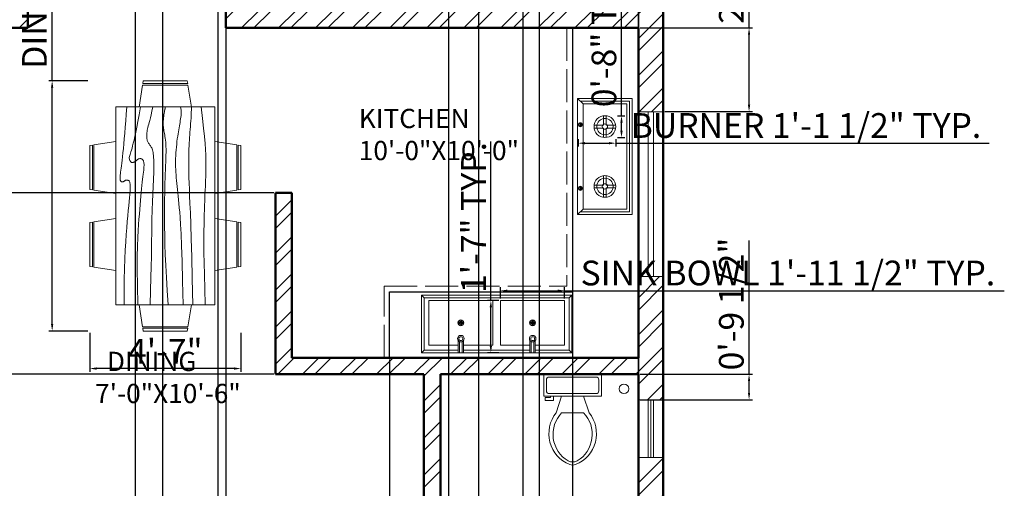
# Model space of a CAD drawing. Units: inches. Extents: x 1104 to 1745, y 678 to 1361.
# Tile 3 of 4: x 1387 to 1745, y 910 to 1080. Entities that reach past the tile are written whole.
import ezdxf

# ---------------------------------------------------------------- set-up
doc = ezdxf.new("R2010")
doc.units = ezdxf.units.IN
doc.linetypes.add('ACAD_ISO02W100', pattern=[15, 12, -3])
for name, color, linetype, lineweight in [('A-ANNO-DIMS', 2, 'Continuous', 18), ('A-AREA-IDEN', 7, 'Continuous', 25), ('A-EQPM', 9, 'Continuous', 18), ('A-FLOR-CASE', 32, 'Continuous', 25), ('A-FLOR-CASE-OVHD', 32, 'ACAD_ISO02W100', 18), ('A-FLOR-FIXT', 8, 'Continuous', 18), ('A-FURN', 8, 'Continuous', 18), ('A-WALL', 7, 'Continuous', 50), ('A-WALL-PATT', 252, 'ACAD_ISO02W100', 13)]:
    doc.layers.add(name, color=color, linetype=linetype, lineweight=lineweight)
doc.layers.add('A-GLAZ', color=244, linetype='Continuous', lineweight=18, true_color=0x991b1e)
doc.styles.get("Standard").update_dxf_attribs({"font": 'arial.ttf'})
doc.dimstyles.new('ISO-25', dxfattribs={"dimtxt": 9, "dimasz": 2.5, "dimexe": 1.25, "dimexo": 0.625, "dimtad": 1, "dimlunit": 3, "dimtxsty": 'Standard', "dimcen": 2.5, "dimadec": 0, "dimazin": 0, "dimtfac": 1, "dimtmove": 0, "dimatfit": 3, "dimfxl": 1, "dimarcsym": 0})

# ---------------------------------------------------------------- blocks, each defined once
blk = doc.blocks.new('*U14')
for p, q in [((9.5, -6), (9.5, -2)), ((-10, -8.5), (-8, -8.5)), ((-10, -9.5), (-10, -8.5)), ((-7, -9.5), (-10, -9.5)), ((-8, -8.5), (-8, -8)), ((-7, -8), (-7, -9.5)), ((-4, -8), (-6, -14)), ((4, -8), (6, -14)), ((4, -14), (-4, -14))]:
    blk.add_line(p, q)
blk.add_lwpolyline([(10.5, -8), (10.5, 0), (-10.5, 0), (-10.5, -8)], close=True)
for points in [[(-9.5, -2), (-9.5, -6)], [(8.5, -1), (-8.5, -1)], [(-8.5, -7), (8.5, -7)]]:
    blk.add_lwpolyline(points)
for centre, radius, start, end in [((-8.62, -1.88), 0.884, 81.8699, 188.1301), ((8.62, -1.88), 0.884, 351.8699, 98.1301), ((-8.62, -6.12), 0.884, 171.8699, 278.1301), ((8.62, -6.12), 0.884, 261.8699, 8.1301), ((3.52, -21.58), 12.17, 141.4691, 247.9714), ((4.2, -21.82), 11.33, 136.3677, 238.9468), ((-3.52, -21.58), 12.17, 292.0284, 38.5307), ((-4.2, -21.82), 11.33, 301.053, 43.6321), ((0, -27.88), 4, 245.7318, 294.2682), ((0, -29), 4, 254.8605, 285.1395)]:
    blk.add_arc(centre, radius, start, end)
blk = doc.blocks.new('Dining Set - 36 x 72 in.')
for p, q in [((-22.2343, 26.00059), (-23.4847, 17.99762)), ((-22.2304, 26), (-5.7608, 26)), ((-22, 27.5), (-22.1562, 26.50042)), ((-5.8416, 26.5), (-22.1534, 26.5)), ((-22, 27.5), (-6, 27.5)), ((-5.8437, 26.49966), (-6, 27.5)), ((-4.5152, 17.99762), (-5.7655, 25.99926)), ((5.7657, 26.00059), (4.5153, 17.99762)), ((5.7696, 26), (22.2392, 26)), ((6, 27.5), (5.8438, 26.50042)), ((22.1584, 26.5), (5.8466, 26.5)), ((6, 27.5), (22, 27.5)), ((22.1563, 26.49966), (22, 27.5)), ((23.4848, 17.99762), (22.2345, 25.99926)), ((36, 18), (-36, 18)), ((-36, 18), (-36, -18)), ((36, -18), (36, 18)), ((-45.5, 8), (-44.5004, 8.15617)), ((-45.5, 8), (-45.5, -8)), ((-44.5, -8.15843), (-44.5, 8.15338)), ((-44.0006, 8.23428), (-35.9976, 9.48474)), ((-44, 8.23041), (-44, -8.23915)), ((44.0006, 8.23428), (35.9976, 9.48474)), ((44, 8.23041), (44, -8.23915)), ((44.5, -8.15843), (44.5, 8.15338)), ((45.5, 8), (44.5005, 8.15617)), ((45.5, 8), (45.5, -8)), ((-44.4997, -8.15631), (-45.5, -8)), ((-35.9976, -9.48476), (-43.9993, -8.2345)), ((35.9976, -9.48476), (43.9993, -8.2345)), ((44.4997, -8.15631), (45.5, -8)), ((-36, -18), (36, -18)), ((-22.2343, -26.0006), (-23.4847, -17.99762)), ((-4.5152, -17.99762), (-5.7655, -25.99928)), ((5.7657, -26.0006), (4.5153, -17.99762)), ((23.4848, -17.99762), (22.2345, -25.99928)), ((-22.2304, -26), (-5.7608, -26)), ((-22, -27.5), (-22.1562, -26.50044)), ((-5.8416, -26.5), (-22.1534, -26.5)), ((-22, -27.5), (-6, -27.5)), ((-5.8437, -26.49967), (-6, -27.5)), ((5.7696, -26), (22.2392, -26)), ((6, -27.5), (5.8438, -26.50044)), ((22.1584, -26.5), (5.8466, -26.5)), ((6, -27.5), (22, -27.5)), ((22.1563, -26.49967), (22, -27.5))]:
    blk.add_line(p, q)
for points in [[(-36, 15), (-31.1772, 14.97754), (-26.8079, 14.91406), (-22.8538, 14.81543), (-19.276, 14.6875), (-16.0362, 14.53613), (-13.0957, 14.36718), (-10.4159, 14.18652), (-7.9583, 14), (-5.6904, 13.81315), (-3.6035, 13.63021), (-1.6954, 13.45508), (0.0365, 13.29166), (1.5945, 13.14388), (2.9811, 13.01562), (4.1988, 12.9108), (5.25, 12.83333), (6.1393, 12.78613), (6.8802, 12.76823), (7.4883, 12.77767), (7.9792, 12.8125), (8.3685, 12.87077), (8.6719, 12.95052), (8.9049, 13.0498), (9.0833, 13.16666), (9.2205, 13.29899), (9.3216, 13.44401), (9.3895, 13.59879), (9.4271, 13.76041), (9.4373, 13.92594), (9.4232, 14.09245), (9.3875, 14.257), (9.3333, 14.41666), (9.2638, 14.56917), (9.1836, 14.71484), (9.0975, 14.85465), (9.0104, 14.98958), (8.9272, 15.1206), (8.8529, 15.2487), (8.7922, 15.37483), (8.75, 15.5), (8.7305, 15.62467), (8.7344, 15.74739), (8.7617, 15.86621), (8.8125, 15.97916), (8.8867, 16.08431), (8.9844, 16.17968), (9.1055, 16.26334), (9.25, 16.33333), (9.4189, 16.38802), (9.6172, 16.42708), (9.8506, 16.45052), (10.125, 16.45833), (10.4463, 16.45052), (10.8203, 16.42708), (11.2529, 16.38802), (11.75, 16.33333), (12.3184, 16.26318), (12.9694, 16.17838), (13.7151, 16.07991), (14.5677, 15.96875), (15.5395, 15.84586), (16.6426, 15.71224), (17.8893, 15.56884), (19.2917, 15.41666), (20.859, 15.25667), (22.5879, 15.08984), (24.4721, 14.91715), (26.5052, 14.73958), (28.6809, 14.5581), (30.9929, 14.3737), (33.4347, 14.18733), (36, 14)], [(-36, 10), (-28.9766, 10.14274), (-23.1725, 10.20442), (-18.4241, 10.19775), (-14.5677, 10.13541), (-11.4399, 10.03011), (-8.877, 9.89453), (-6.7154, 9.74137), (-4.7917, 9.58333), (-2.9698, 9.43082), (-1.2246, 9.28515), (0.4415, 9.14534), (2.026, 9.01041), (3.5266, 8.87939), (4.9408, 8.7513), (6.266, 8.62516), (7.5, 8.5), (8.6411, 8.37549), (9.6914, 8.2539), (10.6538, 8.13818), (11.5312, 8.03125), (12.3267, 7.93603), (13.043, 7.85547), (13.6831, 7.79248), (14.25, 7.75), (14.7471, 7.7303), (15.1797, 7.73307), (15.5537, 7.75732), (15.875, 7.80208), (16.1494, 7.86637), (16.3828, 7.94922), (16.5811, 8.04964), (16.75, 8.16666), (16.8944, 8.29915), (17.0143, 8.44531), (17.1089, 8.60319), (17.1771, 8.77083), (17.218, 8.94629), (17.2305, 9.1276), (17.2137, 9.31282), (17.1667, 9.5), (17.0895, 9.6875), (16.987, 9.875), (16.8649, 10.0625), (16.7292, 10.25), (16.5856, 10.4375), (16.4401, 10.625), (16.2985, 10.8125), (16.1667, 11), (16.05, 11.18733), (15.9518, 11.3737), (15.8752, 11.5581), (15.8229, 11.73958), (15.798, 11.91715), (15.8034, 12.08984), (15.842, 12.25667), (15.9167, 12.41666), (16.0295, 12.56836), (16.1784, 12.70833), (16.3605, 12.83268), (16.5729, 12.9375), (16.8127, 13.01888), (17.0768, 13.07291), (17.3625, 13.0957), (17.6667, 13.08333), (17.9894, 13.03312), (18.3418, 12.94726), (18.7382, 12.82918), (19.1927, 12.68229), (19.7195, 12.51001), (20.3327, 12.31575), (21.0465, 12.10294), (21.875, 11.875), (22.8357, 11.63354), (23.959, 11.37304), (25.2786, 11.08618), (26.8282, 10.76562), (28.6414, 10.40405), (30.752, 9.99414), (33.1936, 9.52856), (36, 9)], [(-36, 5.5), (-30.7157, 5.3348), (-26.069, 5.20963), (-21.9946, 5.11767), (-18.4271, 5.05208), (-15.3009, 5.00602), (-12.5508, 4.97265), (-10.1112, 4.94515), (-7.9167, 4.91666), (-5.909, 4.88167), (-4.0586, 4.83984), (-2.3429, 4.79215), (-0.7396, 4.73958), (0.7739, 4.6831), (2.22, 4.6237), (3.6213, 4.56233), (5, 4.5), (6.373, 4.43782), (7.7344, 4.3776), (9.0723, 4.32129), (10.375, 4.27083), (11.6309, 4.22819), (12.8281, 4.19531), (13.9551, 4.17415), (15, 4.16666), (15.954, 4.17448), (16.819, 4.19791), (17.6001, 4.23698), (18.3021, 4.29166), (18.9299, 4.36198), (19.4883, 4.44791), (19.9823, 4.54948), (20.4167, 4.66666), (20.7969, 4.79899), (21.1302, 4.94401), (21.4245, 5.09879), (21.6875, 5.26041), (21.9271, 5.42594), (22.1511, 5.59245), (22.3672, 5.757), (22.5834, 5.91666), (22.8065, 6.06868), (23.0404, 6.21093), (23.2879, 6.34147), (23.5521, 6.45833), (23.8358, 6.55957), (24.142, 6.64323), (24.4735, 6.70735), (24.8334, 6.75), (25.2235, 6.76969), (25.642, 6.76692), (26.0858, 6.74267), (26.5521, 6.69791), (27.0379, 6.63362), (27.5404, 6.55078), (28.0565, 6.45036), (28.5834, 6.33333), (29.1242, 6.19987), (29.7071, 6.04687), (30.3661, 5.87044), (31.1354, 5.66666), (32.0493, 5.43164), (33.142, 5.16146), (34.4475, 4.85221), (36, 4.5)], [(-36, -1), (-30.7915, -0.6591), (-26.0195, -0.38216), (-21.6519, -0.16284), (-17.6563, 0.00521), (-14.0005, 0.12833), (-10.6523, 0.21289), (-7.5796, 0.26522), (-4.75, 0.29166), (-2.134, 0.29793), (0.2878, 0.28711), (2.5317, 0.26163), (4.6146, 0.22396), (6.5529, 0.17651), (8.3633, 0.12174), (10.0623, 0.06209), (11.6667, 0), (13.1899, -0.06201), (14.6341, -0.1211), (15.9982, -0.17432), (17.2813, -0.21875), (18.4823, -0.25147), (19.6003, -0.26953), (20.6343, -0.27002), (21.5834, -0.25), (22.4481, -0.20768), (23.2357, -0.14584), (23.9549, -0.06836), (24.6146, 0.02083), (25.2235, 0.11784), (25.7904, 0.21875), (26.3241, 0.31966), (26.8334, 0.41666), (27.3265, 0.50618), (27.8099, 0.58593), (28.2894, 0.65397), (28.7709, 0.70833), (29.2601, 0.74707), (29.763, 0.76823), (30.2855, 0.76985), (30.8334, 0.75), (31.4088, 0.70784), (31.9994, 0.64713), (32.589, 0.57275), (33.1615, 0.48958), (33.7008, 0.4025), (34.1908, 0.3164), (34.6153, 0.23616), (34.9584, 0.16666), (35.2099, 0.11165), (35.3848, 0.07031), (35.504, 0.04069), (35.5886, 0.02083), (35.6594, 0.00879), (35.7377, 0.0026), (35.8442, 0.00032), (36, 0)], [(-36, -6.5), (-27.1843, -6.31267), (-20.084, -6.1263), (-14.469, -5.9419), (-10.1094, -5.76042), (-6.7752, -5.58285), (-4.2363, -5.41016), (-2.2629, -5.24333), (-0.625, -5.08334), (0.8708, -4.93099), (2.2715, -4.78646), (3.5872, -4.64974), (4.8281, -4.52084), (6.0046, -4.39974), (7.127, -4.28646), (8.2053, -4.18099), (9.25, -4.08334), (10.2705, -3.99382), (11.2734, -3.91407), (12.2647, -3.84603), (13.25, -3.79167), (14.2354, -3.75293), (15.2266, -3.73177), (16.2295, -3.73015), (17.25, -3.75), (18.2912, -3.79248), (19.3451, -3.85547), (20.4009, -3.93604), (21.4479, -4.03125), (22.4754, -4.13819), (23.4727, -4.25391), (24.4289, -4.37549), (25.3334, -4.5), (26.1785, -4.62492), (26.9694, -4.74935), (27.7145, -4.87281), (28.4219, -4.99479), (29.1, -5.11483), (29.7572, -5.23242), (30.4016, -5.34709), (31.0417, -5.45834), (31.6837, -5.56437), (32.3262, -5.65821), (32.9658, -5.73153), (33.599, -5.77604), (34.2224, -5.78345), (34.8327, -5.74545), (35.4264, -5.65373), (36, -5.5)], [(-36, -10), (-26.4022, -9.81299), (-18.4675, -9.62891), (-11.9839, -9.45069), (-6.7396, -9.28125), (-2.5226, -9.12354), (0.8789, -8.98047), (3.6769, -8.85498), (6.0833, -8.75), (8.2767, -8.66765), (10.3021, -8.60677), (12.1712, -8.56543), (13.8958, -8.54167), (15.4876, -8.53353), (16.9583, -8.53907), (18.3197, -8.55632), (19.5834, -8.58334), (20.7616, -8.61841), (21.8685, -8.66081), (22.9188, -8.71004), (23.9271, -8.76563), (24.9081, -8.82707), (25.8763, -8.89388), (26.8465, -8.96558), (27.8334, -9.04167), (28.8474, -9.12118), (29.8828, -9.20117), (30.93, -9.27824), (31.9792, -9.34896), (33.0205, -9.40991), (34.0443, -9.45768), (35.0407, -9.48885), (36, -9.5)], [(-36, -14.5), (-30.0881, -14.33513), (-25.0332, -14.21224), (-20.7312, -14.12647), (-17.0781, -14.07292), (-13.97, -14.04671), (-11.3027, -14.04297), (-8.9724, -14.05681), (-6.875, -14.08334), (-4.9224, -14.11833), (-3.0905, -14.16016), (-1.3709, -14.20785), (0.2448, -14.26042), (1.7647, -14.3169), (3.1973, -14.3763), (4.5507, -14.43767), (5.8333, -14.5), (7.0554, -14.5621), (8.235, -14.62175), (9.3922, -14.67652), (10.5469, -14.72396), (11.7192, -14.76164), (12.929, -14.78711), (14.1965, -14.79794), (15.5417, -14.79167), (16.9933, -14.76424), (18.6152, -14.70508), (20.4804, -14.60197), (22.6615, -14.44271), (25.2312, -14.21509), (28.2624, -13.9069), (31.8277, -13.50594), (36, -13)]]:
    blk.add_lwpolyline(points)
blk = doc.blocks.new('WIN-GLASS-60IN')
for p, q in [((0, 2), (60, 2)), ((0, 0), (60, 0))]:
    blk.add_line(p, q)
blk = doc.blocks.new('WIN-GLASS-21IN')
for p, q in [((0, 2), (21, 2)), ((0, 1), (21, 1)), ((0, 0), (21, 0))]:
    blk.add_line(p, q)
blk = doc.blocks.new('COOKTOP-BURNER-WITH-CONTROL')
for p, q in [((9.22, 7.94), (9.22, 4.47)), ((10.22, 7.94), (10.22, 4.47)), ((0.54, 5.28), (0.54, 4.06)), ((0.94, 5.28), (0.94, 4.06)), ((5.74, 4.47), (9.22, 4.47)), ((10.22, 4.47), (13.69, 4.47)), ((5.74, 3.47), (9.22, 3.47)), ((9.22, 3.47), (9.22, 0)), ((10.22, 3.47), (10.22, 0)), ((10.22, 3.47), (13.69, 3.47))]:
    blk.add_line(p, q)
for centre, radius in [((9.72, 3.97), 3.97), ((0.74, 4.67), 0.738), ((0.74, 4.67), 0.638), ((9.72, 3.97), 2.97), ((9.72, 3.97), 0.972)]:
    blk.add_circle(centre, radius)
blk = doc.blocks.new('SINK-BOWL-WITH-TAP')
for p, q in [((10.62, 11.12), (12.72, 11.12)), ((11.47, 11.98), (11.47, 9.87)), ((11.87, 11.98), (11.87, 9.87)), ((10.62, 10.72), (12.72, 10.72)), ((10.67, 0), (10.67, 4.54)), ((11.17, 0), (11.17, 4.07)), ((12.17, 0), (12.17, 4.03)), ((12.67, 0), (12.67, 4.42))]:
    blk.add_line(p, q)
blk.add_lwpolyline([(10.67, 2.77), (0, 2.77), (0, 19.08), (23.33, 19.08), (23.33, 2.77), (12.67, 2.77)])
for centre, radius in [((11.67, 10.92), 1.07), ((11.67, 10.92), 0.569), ((11.7, 5.14), 1.2), ((11.7, 5.14), 0.703)]:
    blk.add_circle(centre, radius)
blk = doc.blocks.new('*D27')
at = {"layer": 'A-ANNO-DIMS', "color": 0, "lineweight": -2, "transparency": 16777216}
for p, q in [((1590.21, 1036.62), (1590.21, 1033.95)), ((1592.71, 1035.2), (1601.4, 1035.2)), ((1603.9, 1036.62), (1603.9, 1033.95)), ((1603.9, 1035.2), (1739.66, 1035.2))]:
    blk.add_line(p, q, dxfattribs=at)
at = {"layer": 'A-ANNO-DIMS', "color": 0, "transparency": 16777216}
for points in [[(1592.71, 1035.61), (1592.71, 1034.78), (1590.21, 1035.2)], [(1601.4, 1035.61), (1601.4, 1034.78), (1603.9, 1035.2)]]:
    blk.add_solid(points, dxfattribs=at)
at = {"layer": 'Defpoints', "color": 0, "transparency": 16777216}
for p in [(1590.21, 1037.25), (1603.9, 1037.25), (1603.9, 1035.2)]:
    blk.add_point(p, dxfattribs=at)
at = {"layer": 'A-ANNO-DIMS', "color": 0, "transparency": 16777216, "insert": (1673.03, 1040.47), "char_height": 9, "attachment_point": 5}
blk.add_mtext('BURNER 1\'-1 1/2" TYP.', dxfattribs=at)
blk = doc.blocks.new('*D28')
at = {"layer": 'A-ANNO-DIMS', "color": 0, "lineweight": -2, "transparency": 16777216}
for p, q in [((1605.95, 1045.19), (1605.95, 1103.8)), ((1604.52, 1045.19), (1607.2, 1045.19)), ((1605.95, 1039.75), (1605.95, 1042.69)), ((1604.52, 1037.25), (1607.2, 1037.25))]:
    blk.add_line(p, q, dxfattribs=at)
at = {"layer": 'A-ANNO-DIMS', "color": 0, "transparency": 16777216}
for points in [[(1605.53, 1042.69), (1606.37, 1042.69), (1605.95, 1045.19)], [(1605.53, 1039.75), (1606.37, 1039.75), (1605.95, 1037.25)]]:
    blk.add_solid(points, dxfattribs=at)
at = {"layer": 'Defpoints', "color": 0, "transparency": 16777216}
for p in [(1603.9, 1045.19), (1605.95, 1045.19), (1603.9, 1037.25)]:
    blk.add_point(p, dxfattribs=at)
at = {"layer": 'A-ANNO-DIMS', "color": 0, "transparency": 16777216, "insert": (1600.73, 1075.75), "char_height": 9, "attachment_point": 5, "rotation": 90}
blk.add_mtext('0\'-8" TYP.', dxfattribs=at)
blk = doc.blocks.new('*D29')
at = {"layer": 'A-ANNO-DIMS', "color": 0, "lineweight": -2, "transparency": 16777216}
for p, q in [((1561.94, 978.65), (1561.94, 982.78)), ((1564.44, 981.53), (1582.78, 981.53)), ((1585.28, 978.65), (1585.28, 982.78)), ((1585.28, 981.53), (1745.16, 981.53))]:
    blk.add_line(p, q, dxfattribs=at)
at = {"layer": 'A-ANNO-DIMS', "color": 0, "transparency": 16777216}
for points in [[(1564.44, 981.94), (1564.44, 981.11), (1561.94, 981.53)], [(1582.78, 981.94), (1582.78, 981.11), (1585.28, 981.53)]]:
    blk.add_solid(points, dxfattribs=at)
at = {"layer": 'Defpoints', "color": 0, "transparency": 16777216}
for p in [(1585.28, 981.53), (1561.94, 978.03), (1585.28, 978.03)]:
    blk.add_point(p, dxfattribs=at)
at = {"layer": 'A-ANNO-DIMS', "color": 0, "transparency": 16777216, "insert": (1666.47, 986.81), "char_height": 9, "attachment_point": 5}
blk.add_mtext('SINK BOWL 1\'-11 1/2" TYP.', dxfattribs=at)
blk = doc.blocks.new('*D30')
at = {"layer": 'A-ANNO-DIMS', "color": 0, "lineweight": -2, "transparency": 16777216}
for p, q in [((1558.45, 978.03), (1558.45, 1035.79)), ((1561.32, 978.03), (1557.2, 978.03)), ((1558.45, 961.45), (1558.45, 975.53)), ((1561.32, 958.95), (1557.2, 958.95))]:
    blk.add_line(p, q, dxfattribs=at)
at = {"layer": 'A-ANNO-DIMS', "color": 0, "transparency": 16777216}
for points in [[(1558.03, 975.53), (1558.86, 975.53), (1558.45, 978.03)], [(1558.03, 961.45), (1558.86, 961.45), (1558.45, 958.95)]]:
    blk.add_solid(points, dxfattribs=at)
at = {"layer": 'Defpoints', "color": 0, "transparency": 16777216}
for p in [(1558.45, 978.03), (1561.94, 978.03), (1561.94, 958.95)]:
    blk.add_point(p, dxfattribs=at)
at = {"layer": 'A-ANNO-DIMS', "color": 0, "transparency": 16777216, "insert": (1553.3, 1008.16), "char_height": 9, "attachment_point": 5, "rotation": 90}
blk.add_mtext('1\'-7" TYP.', dxfattribs=at)
blk = doc.blocks.new('*D31')
at = {"layer": 'A-ANNO-DIMS', "color": 0, "lineweight": -2, "transparency": 16777216}
for p, q in [((1398.91, 1057.87), (1398.91, 1160.54)), ((1411.93, 1057.87), (1397.66, 1057.87)), ((1398.91, 969.37), (1398.91, 1055.37)), ((1411.93, 966.87), (1397.66, 966.87))]:
    blk.add_line(p, q, dxfattribs=at)
at = {"layer": 'A-ANNO-DIMS', "color": 0, "transparency": 16777216}
for points in [[(1398.49, 1055.37), (1399.32, 1055.37), (1398.91, 1057.87)], [(1398.49, 969.37), (1399.32, 969.37), (1398.91, 966.87)]]:
    blk.add_solid(points, dxfattribs=at)
at = {"layer": 'Defpoints', "color": 0, "transparency": 16777216}
for p in [(1398.91, 1057.87), (1412.56, 1057.87), (1412.56, 966.87)]:
    blk.add_point(p, dxfattribs=at)
at = {"layer": 'A-ANNO-DIMS', "color": 0, "transparency": 16777216, "insert": (1393.63, 1110.45), "char_height": 9, "attachment_point": 5, "rotation": 90}
blk.add_mtext('DINING SET 7\'-7"', dxfattribs=at)
blk = doc.blocks.new('*D32')
at = {"layer": 'A-ANNO-DIMS', "color": 0, "lineweight": -2, "transparency": 16777216}
for p, q in [((1412.56, 966.24), (1412.56, 951.97)), ((1467.56, 966.24), (1467.56, 951.97)), ((1465.06, 953.22), (1415.06, 953.22))]:
    blk.add_line(p, q, dxfattribs=at)
at = {"layer": 'A-ANNO-DIMS', "color": 0, "transparency": 16777216}
for points in [[(1415.06, 953.63), (1415.06, 952.8), (1412.56, 953.22)], [(1465.06, 953.63), (1465.06, 952.8), (1467.56, 953.22)]]:
    blk.add_solid(points, dxfattribs=at)
at = {"layer": 'Defpoints', "color": 0, "transparency": 16777216}
for p in [(1412.56, 966.87), (1467.56, 966.87), (1412.56, 953.22)]:
    blk.add_point(p, dxfattribs=at)
at = {"layer": 'A-ANNO-DIMS', "color": 0, "transparency": 16777216, "insert": (1440.06, 958.34), "char_height": 9, "attachment_point": 5}
blk.add_mtext('4\'-7"', dxfattribs=at)
blk = doc.blocks.new('*D39')
at = {"layer": 'A-ANNO-DIMS', "color": 0, "lineweight": -2, "transparency": 16777216}
for p, q in [((1429.11, 1148.5), (1429.11, 684.69)), ((1459.11, 1148.5), (1459.11, 684.69)), ((1431.61, 685.94), (1456.61, 685.94))]:
    blk.add_line(p, q, dxfattribs=at)
at = {"layer": 'A-ANNO-DIMS', "color": 0, "transparency": 16777216}
for points in [[(1431.61, 686.36), (1431.61, 685.52), (1429.11, 685.94)], [(1456.61, 686.36), (1456.61, 685.52), (1459.11, 685.94)]]:
    blk.add_solid(points, dxfattribs=at)
at = {"layer": 'Defpoints', "color": 0, "transparency": 16777216}
for p in [(1429.11, 1149.13), (1459.11, 1149.13), (1459.11, 685.94)]:
    blk.add_point(p, dxfattribs=at)
at = {"layer": 'A-ANNO-DIMS', "color": 0, "transparency": 16777216, "insert": (1444.11, 691.16), "char_height": 9, "attachment_point": 5}
blk.add_mtext('2\'-6"', dxfattribs=at)
blk = doc.blocks.new('*D42')
at = {"layer": 'A-ANNO-DIMS', "color": 0, "lineweight": -2, "transparency": 16777216}
for p, q in [((1588.11, 1076.5), (1588.11, 684.69)), ((1612.11, 1076.5), (1612.11, 684.69)), ((1590.61, 685.94), (1609.61, 685.94)), ((1612.11, 685.94), (1639.93, 685.94))]:
    blk.add_line(p, q, dxfattribs=at)
at = {"layer": 'A-ANNO-DIMS', "color": 0, "transparency": 16777216}
for points in [[(1590.61, 686.36), (1590.61, 685.52), (1588.11, 685.94)], [(1609.61, 686.36), (1609.61, 685.52), (1612.11, 685.94)]]:
    blk.add_solid(points, dxfattribs=at)
at = {"layer": 'Defpoints', "color": 0, "transparency": 16777216}
for p in [(1588.11, 1077.13), (1612.11, 1077.13), (1612.11, 685.94)]:
    blk.add_point(p, dxfattribs=at)
at = {"layer": 'A-ANNO-DIMS', "color": 0, "transparency": 16777216, "insert": (1627.27, 691.16), "char_height": 9, "attachment_point": 5}
blk.add_mtext('2\'-0"', dxfattribs=at)
blk = doc.blocks.new('*D43')
at = {"layer": 'A-ANNO-DIMS', "color": 0, "lineweight": -2, "transparency": 16777216}
for p, q in [((1521.6, 956.5), (1521.6, 684.69)), ((1612.11, 956.5), (1612.11, 684.69)), ((1524.1, 685.94), (1609.61, 685.94))]:
    blk.add_line(p, q, dxfattribs=at)
at = {"layer": 'A-ANNO-DIMS', "color": 0, "transparency": 16777216}
for points in [[(1524.1, 686.36), (1524.1, 685.52), (1521.6, 685.94)], [(1609.61, 686.36), (1609.61, 685.52), (1612.11, 685.94)]]:
    blk.add_solid(points, dxfattribs=at)
at = {"layer": 'Defpoints', "color": 0, "transparency": 16777216}
for p in [(1521.6, 957.13), (1612.11, 957.13), (1612.11, 685.94)]:
    blk.add_point(p, dxfattribs=at)
at = {"layer": 'A-ANNO-DIMS', "color": 0, "transparency": 16777216, "insert": (1566.85, 691.22), "char_height": 9, "attachment_point": 5}
blk.add_mtext('7\'-6 1/2"', dxfattribs=at)
blk = doc.blocks.new('*D44')
at = {"layer": 'A-ANNO-DIMS', "color": 0, "lineweight": -2, "transparency": 16777216}
for p, q in [((1479.48, 1017.13), (1198.71, 1017.13)), ((1199.96, 1014.63), (1199.96, 953.63)), ((1479.48, 951.13), (1198.71, 951.13))]:
    blk.add_line(p, q, dxfattribs=at)
at = {"layer": 'A-ANNO-DIMS', "color": 0, "transparency": 16777216}
for points in [[(1199.54, 1014.63), (1200.37, 1014.63), (1199.96, 1017.13)], [(1199.54, 953.63), (1200.37, 953.63), (1199.96, 951.13)]]:
    blk.add_solid(points, dxfattribs=at)
at = {"layer": 'Defpoints', "color": 0, "transparency": 16777216}
for p in [(1480.11, 1017.13), (1199.96, 951.13), (1480.11, 951.13)]:
    blk.add_point(p, dxfattribs=at)
at = {"layer": 'A-ANNO-DIMS', "color": 0, "transparency": 16777216, "insert": (1194.74, 984.13), "char_height": 9, "attachment_point": 5, "rotation": 90}
blk.add_mtext('5\'-6"', dxfattribs=at)
blk = doc.blocks.new('*D49')
at = {"layer": 'A-ANNO-DIMS', "color": 0, "lineweight": -2, "transparency": 16777216}
for p, q in [((1652.34, 1077.13), (1652.34, 1125.93)), ((1612.73, 1077.13), (1653.59, 1077.13)), ((1652.34, 1049.17), (1652.34, 1074.63)), ((1621.73, 1046.67), (1653.59, 1046.67))]:
    blk.add_line(p, q, dxfattribs=at)
at = {"layer": 'A-ANNO-DIMS', "color": 0, "transparency": 16777216}
for points in [[(1651.93, 1074.63), (1652.76, 1074.63), (1652.34, 1077.13)], [(1651.93, 1049.17), (1652.76, 1049.17), (1652.34, 1046.67)]]:
    blk.add_solid(points, dxfattribs=at)
at = {"layer": 'Defpoints', "color": 0, "transparency": 16777216}
for p in [(1612.11, 1077.13), (1652.34, 1077.13), (1621.11, 1046.67)]:
    blk.add_point(p, dxfattribs=at)
at = {"layer": 'A-ANNO-DIMS', "color": 0, "transparency": 16777216, "insert": (1647.06, 1102.78), "char_height": 9, "attachment_point": 5, "rotation": 90}
blk.add_mtext('2\'-6 1/2"', dxfattribs=at)
blk = doc.blocks.new('*D50')
at = {"layer": 'A-ANNO-DIMS', "color": 0, "lineweight": -2, "transparency": 16777216}
for p, q in [((1652.34, 951.13), (1652.34, 999.77)), ((1612.73, 951.13), (1653.59, 951.13)), ((1652.34, 944.36), (1652.34, 948.63)), ((1612.73, 941.86), (1653.59, 941.86))]:
    blk.add_line(p, q, dxfattribs=at)
at = {"layer": 'A-ANNO-DIMS', "color": 0, "transparency": 16777216}
for points in [[(1651.93, 948.63), (1652.76, 948.63), (1652.34, 951.13)], [(1651.93, 944.36), (1652.76, 944.36), (1652.34, 941.86)]]:
    blk.add_solid(points, dxfattribs=at)
at = {"layer": 'Defpoints', "color": 0, "transparency": 16777216}
for p in [(1612.11, 951.13), (1652.34, 951.13), (1612.11, 941.86)]:
    blk.add_point(p, dxfattribs=at)
at = {"layer": 'A-ANNO-DIMS', "color": 0, "transparency": 16777216, "insert": (1647.06, 976.7), "char_height": 9, "attachment_point": 5, "rotation": 90}
blk.add_mtext('0\'-9 1/2"', dxfattribs=at)
blk = doc.blocks.new('*D53')
at = {"layer": 'A-ANNO-DIMS', "color": 0, "lineweight": -2, "transparency": 16777216}
for p, q in [((1576.11, 741.75), (1576.11, 1343.53)), ((1612.11, 741.75), (1612.11, 1343.53)), ((1578.61, 1342.28), (1609.61, 1342.28))]:
    blk.add_line(p, q, dxfattribs=at)
at = {"layer": 'A-ANNO-DIMS', "color": 0, "transparency": 16777216}
for points in [[(1578.61, 1342.7), (1578.61, 1341.86), (1576.11, 1342.28)], [(1609.61, 1342.7), (1609.61, 1341.86), (1612.11, 1342.28)]]:
    blk.add_solid(points, dxfattribs=at)
at = {"layer": 'Defpoints', "color": 0, "transparency": 16777216}
for p in [(1612.11, 1342.28), (1576.11, 741.13), (1612.11, 741.13)]:
    blk.add_point(p, dxfattribs=at)
at = {"layer": 'A-ANNO-DIMS', "color": 0, "transparency": 16777216, "insert": (1594.11, 1347.5), "char_height": 9, "attachment_point": 5}
blk.add_mtext('3\'-0"', dxfattribs=at)
blk = doc.blocks.new('*D55')
at = {"layer": 'A-ANNO-DIMS', "color": 0, "lineweight": -2, "transparency": 16777216}
for p, q in [((1543.11, 819.75), (1543.11, 1343.53)), ((1554.11, 819.75), (1554.11, 1343.53)), ((1545.61, 1342.28), (1551.61, 1342.28)), ((1554.11, 1342.28), (1588.77, 1342.28))]:
    blk.add_line(p, q, dxfattribs=at)
at = {"layer": 'A-ANNO-DIMS', "color": 0, "transparency": 16777216}
for points in [[(1545.61, 1342.7), (1545.61, 1341.86), (1543.11, 1342.28)], [(1551.61, 1342.7), (1551.61, 1341.86), (1554.11, 1342.28)]]:
    blk.add_solid(points, dxfattribs=at)
at = {"layer": 'Defpoints', "color": 0, "transparency": 16777216}
for p in [(1554.11, 1342.28), (1543.11, 819.13), (1554.11, 819.13)]:
    blk.add_point(p, dxfattribs=at)
at = {"layer": 'A-ANNO-DIMS', "color": 0, "transparency": 16777216, "insert": (1572.69, 1347.5), "char_height": 9, "attachment_point": 5}
blk.add_mtext('0\'-11"', dxfattribs=at)
blk = doc.blocks.new('*D57')
at = {"layer": 'A-ANNO-DIMS', "color": 0, "lineweight": -2, "transparency": 16777216}
for p, q in [((1439.05, 1250.5), (1439.05, 684.69)), ((1462.11, 1250.5), (1462.11, 684.69)), ((1441.55, 685.94), (1459.61, 685.94)), ((1462.11, 685.94), (1495.93, 685.94))]:
    blk.add_line(p, q, dxfattribs=at)
at = {"layer": 'A-ANNO-DIMS', "color": 0, "transparency": 16777216}
for points in [[(1441.55, 686.36), (1441.55, 685.52), (1439.05, 685.94)], [(1459.61, 686.36), (1459.61, 685.52), (1462.11, 685.94)]]:
    blk.add_solid(points, dxfattribs=at)
at = {"layer": 'Defpoints', "color": 0, "transparency": 16777216}
for p in [(1439.05, 1251.13), (1462.11, 1251.13), (1462.11, 685.94)]:
    blk.add_point(p, dxfattribs=at)
at = {"layer": 'A-ANNO-DIMS', "color": 0, "transparency": 16777216, "insert": (1480.27, 691.08), "char_height": 9, "attachment_point": 5}
blk.add_mtext('1\'-11"', dxfattribs=at)
blk = doc.blocks.new('*D58')
at = {"layer": 'A-ANNO-DIMS', "color": 0, "lineweight": -2, "transparency": 16777216}
for p, q in [((1570.11, 1250.5), (1570.11, 684.69)), ((1612.11, 1250.5), (1612.11, 684.69)), ((1572.61, 685.94), (1609.61, 685.94))]:
    blk.add_line(p, q, dxfattribs=at)
at = {"layer": 'A-ANNO-DIMS', "color": 0, "transparency": 16777216}
for points in [[(1572.61, 686.36), (1572.61, 685.52), (1570.11, 685.94)], [(1609.61, 686.36), (1609.61, 685.52), (1612.11, 685.94)]]:
    blk.add_solid(points, dxfattribs=at)
at = {"layer": 'Defpoints', "color": 0, "transparency": 16777216}
for p in [(1570.11, 1251.13), (1612.11, 1251.13), (1612.11, 685.94)]:
    blk.add_point(p, dxfattribs=at)
at = {"layer": 'A-ANNO-DIMS', "color": 0, "transparency": 16777216, "insert": (1591.11, 691.16), "char_height": 9, "attachment_point": 5}
blk.add_mtext('3\'-6"', dxfattribs=at)

msp = doc.modelspace()

# ---------------------------------------------------------------- hatches: boundary and pattern name
at = {"layer": 'A-WALL-PATT'}
h = msp.add_hatch(dxfattribs=at)
h.set_pattern_fill('ANSI32', color=256)
h.paths.add_polyline_path([(1277.606, 917.921), (1240.106, 917.921), (1240.106, 980.462), (1231.106, 980.462), (1231.106, 719.949), (1240.106, 719.949), (1240.106, 908.921), (1277.606, 908.921)])
h.paths.add_polyline_path([(1384.106, 917.921), (1337.606, 917.921), (1337.606, 908.921), (1375.106, 908.921), (1375.106, 836.921), (1387.106, 836.921), (1387.106, 844.121), (1387.106, 845.921), (1384.106, 845.921)])
h.paths.add_polyline_path([(1486.106, 849.129), (1543.106, 849.129), (1543.106, 855.129), (1540.106, 855.129), (1540.106, 951.129), (1612.106, 951.129), (1612.106, 941.864), (1621.106, 941.864), (1621.106, 986.665), (1612.106, 986.665), (1612.106, 957.129), (1486.106, 957.129), (1486.106, 1017.129), (1480.106, 1017.129), (1480.106, 951.129), (1534.106, 951.129), (1534.106, 855.129), (1480.106, 855.129), (1480.106, 845.921), (1476.166, 845.921), (1476.166, 836.921), (1480.106, 836.921), (1480.106, 833.921), (1486.106, 833.921)])
h.paths.add_polyline_path([(1441.89, 845.921), (1435.106, 845.921), (1435.106, 836.921), (1441.89, 836.921)])
h.paths.add_polyline_path([(1240.106, 1137.841), (1231.106, 1137.841), (1231.106, 1040.462), (1240.106, 1040.462), (1240.106, 1077.129), (1390.106, 1077.129), (1390.106, 1086.129), (1384.106, 1086.129), (1384.106, 1083.129), (1240.106, 1083.129)])
h.paths.add_polyline_path([(1621.106, 1146.091), (1612.106, 1146.091), (1612.106, 1083.129), (1468.106, 1083.129), (1468.106, 1086.129), (1462.106, 1086.129), (1462.106, 1077.129), (1480.106, 1077.129), (1612.106, 1077.129), (1612.106, 1046.665), (1621.106, 1046.665)])
h.paths.add_polyline_path([(1240.106, 1251.129), (1282.106, 1251.129), (1282.106, 1260.129), (1231.106, 1260.129), (1231.106, 1197.841), (1240.106, 1197.841)])
h.paths.add_polyline_path([(1418.05, 1260.129), (1342.106, 1260.129), (1342.106, 1251.129), (1384.106, 1251.129), (1384.106, 1122.129), (1390.106, 1122.129), (1390.106, 1149.129), (1429.106, 1149.129), (1429.106, 1155.129), (1390.106, 1155.129), (1390.106, 1251.129), (1418.05, 1251.129)])
h.paths.add_polyline_path([(1510.106, 1260.129), (1439.05, 1260.129), (1439.05, 1251.129), (1462.106, 1251.129), (1462.106, 1155.129), (1459.106, 1155.129), (1459.106, 1153.629), (1459.106, 1149.129), (1462.106, 1149.129), (1462.106, 1122.129), (1468.106, 1122.129), (1468.106, 1251.129), (1510.106, 1251.129)])
h.paths.add_polyline_path([(1621.106, 1260.129), (1570.106, 1260.129), (1570.106, 1251.129), (1612.106, 1251.129), (1612.106, 1206.091), (1621.106, 1206.091)])
h.paths.add_polyline_path([(1621.106, 920.864), (1612.106, 920.864), (1612.106, 855.129), (1573.106, 855.129), (1573.106, 849.129), (1612.106, 849.129), (1612.106, 809.56), (1621.106, 809.56)])
h.paths.add_polyline_path([(1621.106, 749.56), (1612.106, 749.56), (1612.106, 741.129), (1486.106, 741.129), (1486.106, 797.921), (1480.106, 797.921), (1480.106, 732.129), (1621.106, 732.129)])

# ---------------------------------------------------------------- linework, layer by layer
at = {"layer": 'A-EQPM'}
for p, q in [((1591.965, 1049.482), (1589.965, 1051.482)), ((1591.965, 1011.217), (1589.965, 1009.217))]:
    msp.add_line(p, q, dxfattribs=at)
for points in [[(1589.965, 1051.482), (1609.853, 1051.482), (1609.853, 1009.217), (1589.965, 1009.217)], [(1591.965, 1049.482), (1607.853, 1049.482), (1607.853, 1011.217), (1591.965, 1011.217)]]:
    msp.add_lwpolyline(points, close=True, dxfattribs=at)
msp.add_lwpolyline([(1590.965, 1050.482), (1608.853, 1050.482), (1608.853, 1010.217), (1590.965, 1010.217)], dxfattribs=at)
at = {"layer": 'A-FLOR-CASE'}
for p, q in [((1588.106, 1077.129), (1588.106, 981.129)), ((1521.602, 981.129), (1588.106, 981.129)), ((1521.602, 957.129), (1521.602, 981.129))]:
    msp.add_line(p, q, dxfattribs=at)
at = {"layer": 'A-FLOR-CASE-OVHD'}
for p, q in [((1586.106, 1077.129), (1586.106, 983.129)), ((1519.602, 983.129), (1586.106, 983.129)), ((1519.602, 957.129), (1519.602, 983.129))]:
    msp.add_line(p, q, dxfattribs=at)
at = {"layer": 'A-FLOR-FIXT'}
for p, q in [((1533.227, 979.972), (1534.227, 978.972)), ((1586.92, 978.972), (1587.92, 979.972)), ((1533.227, 958.95), (1534.227, 959.95)), ((1586.92, 959.95), (1587.92, 958.95))]:
    msp.add_line(p, q, dxfattribs=at)
msp.add_lwpolyline([(1533.227, 979.972), (1587.92, 979.972), (1587.92, 958.95), (1533.227, 958.95)], close=True, dxfattribs=at)
for points in [[(1546.535, 959.95), (1534.227, 959.95), (1534.227, 978.972), (1586.92, 978.972), (1586.92, 959.95), (1574.611, 959.95)], [(1572.611, 959.95), (1548.535, 959.95)]]:
    msp.add_lwpolyline(points, dxfattribs=at)
msp.add_circle((1606.856, 945.841), 1.735, dxfattribs=at)
at = {"layer": 'A-GLAZ'}
for points in [[(1621.106, 1046.665), (1621.106, 986.665), (1612.106, 986.665), (1612.106, 1046.665)], [(1612.106, 920.864), (1612.106, 941.864), (1621.106, 941.864), (1621.106, 920.864)]]:
    msp.add_lwpolyline(points, close=True, dxfattribs=at)
at = {"layer": 'A-WALL'}
for p, q in [((1621.106, 1260.129), (1621.106, 732.129)), ((1390.106, 1086.129), (1390.106, 1077.129)), ((1462.106, 1086.129), (1462.106, 1077.129)), ((1240.106, 1077.129), (1390.106, 1077.129)), ((1462.106, 1077.129), (1480.106, 1077.129)), ((1480.106, 1077.129), (1612.106, 1077.129)), ((1612.106, 1077.129), (1612.106, 957.129)), ((1480.106, 1017.129), (1480.106, 951.129)), ((1486.106, 1017.129), (1480.106, 1017.129)), ((1486.106, 1017.129), (1486.106, 957.129)), ((1486.106, 957.129), (1612.106, 957.129)), ((1480.106, 951.129), (1534.106, 951.129)), ((1534.106, 951.129), (1534.106, 855.129)), ((1540.106, 951.129), (1540.106, 855.129)), ((1540.106, 951.129), (1612.106, 951.129)), ((1612.106, 951.129), (1612.106, 855.129))]:
    msp.add_line(p, q, dxfattribs=at)

# ---------------------------------------------------------------- block references
at = {"layer": 'A-EQPM'}
msp.add_blockref('COOKTOP-BURNER-WITH-CONTROL', (1590.209, 1037.25), dxfattribs=at)
at = {"layer": 'A-EQPM', "extrusion": (0, 0, -1), "zscale": -1, "rotation": 180}
msp.add_blockref('COOKTOP-BURNER-WITH-CONTROL', (-1590.209, 1023.449), dxfattribs=at)
at = {"layer": 'A-FLOR-FIXT', "extrusion": (0, 0, -1), "zscale": -1}
msp.add_blockref('SINK-BOWL-WITH-TAP', (-1559.201, 958.95), dxfattribs=at)
at = {"layer": 'A-FLOR-FIXT'}
for name, p in [('SINK-BOWL-WITH-TAP', (1561.945, 958.95)), ('*U14', (1588.192, 951.129))]:
    msp.add_blockref(name, p, dxfattribs=at)
at = {"layer": 'A-FURN', "rotation": 90}
msp.add_blockref('Dining Set - 36 x 72 in.', (1440.056, 1012.365), dxfattribs=at)
at = {"layer": 'A-GLAZ'}
for name, p, rotation in [('WIN-GLASS-60IN', (1615.607, 1046.666), 269.9999999999992), ('WIN-GLASS-21IN', (1617.606, 920.864), 89.99999999999754)]:
    msp.add_blockref(name, p, dxfattribs=dict(at, rotation=rotation))

# ---------------------------------------------------------------- texts
at = {"layer": 'A-AREA-IDEN', "char_height": 7, "attachment_point": 1}
for s, width, insert in [('KITCHEN 10\'-0"X10\'-0"', 54.72096, (1510.426, 1047.693)), ('  DINING 7\'-0"X10\'-6"', 45.74279, (1414.536, 959.319))]:
    msp.add_mtext_dynamic_manual_height_columns(s, width=width, gutter_width=12.5, heights=[0], dxfattribs=dict(at, insert=insert))

# ---------------------------------------------------------------- dimensions: what is measured, and where the dimension line sits
at = {"layer": 'A-ANNO-DIMS'}
for base, p1, p2, picture, middle in [((1554.106, 1342.279), (1543.106, 819.129), (1554.106, 819.129), '*D55', (1572.69, 1347.499)), ((1612.106, 1342.279), (1576.106, 741.129), (1612.106, 741.129), '*D53', (1594.106, 1347.502)), ((1462.106, 685.941), (1439.05, 1251.129), (1462.106, 1251.129), '*D57', (1480.266, 691.084)), ((1612.106, 685.941), (1570.106, 1251.129), (1612.106, 1251.129), '*D58', (1591.106, 691.164)), ((1459.106, 685.941), (1429.106, 1149.129), (1459.106, 1149.129), '*D39', (1444.106, 691.161)), ((1612.106, 685.941), (1588.106, 1077.129), (1612.106, 1077.129), '*D42', (1627.27, 691.161)), ((1612.106, 685.941), (1521.602, 957.129), (1612.106, 957.129), '*D43', (1566.854, 691.219))]:
    dim = msp.add_linear_dim(base=base, p1=p1, p2=p2, dimstyle='ISO-25', override={"dimdec": 1, "dimlfac": 1, "dimrnd": 0, "dimzin": 1, "dimdsep": 46, "dimlunit": 4, "dimfrac": 2}, dxfattribs=at)
    dim.commit()
    dim.dimension.update_dxf_attribs({"geometry": picture, "text_midpoint": middle})
for base, p1, p2, text, picture, middle in [((1398.906, 1057.865), (1412.556, 966.865), (1412.556, 1057.865), 'DINING SET <>', '*D31', (1393.627, 1110.45)), ((1605.95, 1045.194), (1603.897, 1037.25), (1603.897, 1045.194), '<> TYP.', '*D28', (1600.73, 1075.749)), ((1558.445, 978.027), (1561.945, 958.95), (1561.945, 978.027), '<> TYP.', '*D30', (1553.299, 1008.158))]:
    dim = msp.add_linear_dim(base=base, p1=p1, p2=p2, angle=90, text=text, dimstyle='ISO-25', override={"dimdec": 1, "dimlfac": 1, "dimrnd": 0, "dimzin": 1, "dimdsep": 46, "dimlunit": 4, "dimfrac": 2}, dxfattribs=at)
    dim.commit()
    dim.dimension.update_dxf_attribs({"geometry": picture, "text_midpoint": middle})
for base, p1, p2, angle, picture, middle in [((1652.342, 1077.129), (1621.106, 1046.665), (1612.106, 1077.129), 90, '*D49', (1647.064, 1102.778)), ((1199.956, 951.129), (1480.106, 1017.129), (1480.106, 951.129), 90, '*D44', (1194.736, 984.129)), ((1652.342, 951.129), (1612.106, 941.864), (1612.106, 951.129), 90, '*D50', (1647.064, 976.701)), ((1412.556, 953.215), (1467.556, 966.865), (1412.556, 966.865), 180, '*D32', (1440.056, 958.34))]:
    dim = msp.add_linear_dim(base=base, p1=p1, p2=p2, angle=angle, dimstyle='ISO-25', override={"dimdec": 1, "dimlfac": 1, "dimrnd": 0, "dimzin": 1, "dimdsep": 46, "dimlunit": 4, "dimfrac": 2}, dxfattribs=at)
    dim.commit()
    dim.dimension.update_dxf_attribs({"geometry": picture, "text_midpoint": middle})
for base, p1, p2, text, picture, middle in [((1603.897, 1035.196), (1590.209, 1037.25), (1603.897, 1037.25), 'BURNER <> TYP.', '*D27', (1673.03, 1040.475)), ((1585.277, 981.526), (1561.945, 978.027), (1585.277, 978.027), 'SINK BOWL <> TYP.', '*D29', (1666.47, 986.808))]:
    dim = msp.add_linear_dim(base=base, p1=p1, p2=p2, text=text, dimstyle='ISO-25', override={"dimdec": 1, "dimlfac": 1, "dimrnd": 0, "dimzin": 1, "dimdsep": 46, "dimlunit": 4, "dimfrac": 2}, dxfattribs=at)
    dim.commit()
    dim.dimension.update_dxf_attribs({"geometry": picture, "text_midpoint": middle})

doc.saveas('drawing.dxf')
